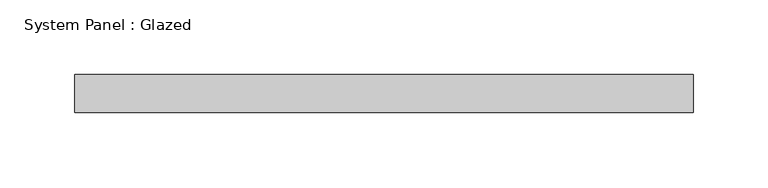
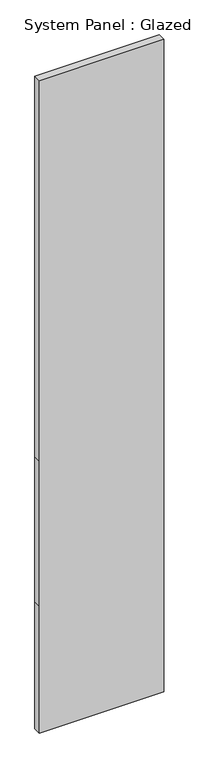
"""IFC4 building model written with IfcOpenShell, lengths in millimetres: plate geometry, System Panel : Glazed."""

from ifc_helpers import new_model, si_unit, frame, origin, place, context, project, spatial, polyline, outline, extrude, source, transform, mapped, element, save


def system_panel_glazed_01ea813e(model_context):
    return source(origin(), model_context, "Body", "SweptSolid", [
        extrude(outline(polyline([(0.0, -206.375), (0.0, 206.375), (444.5, 206.375), (952.5, 206.375), (2286.0, 206.375), (2286.0, -206.375), (952.5, -206.375), (444.5, -206.375), (0.0, -206.375)])), frame((0.0, 19.05, 0.0), z_axis=(0.0, 1.0, 0.0), x_axis=(0.0, 0.0, 1.0)), (0.0, 0.0, 1.0), 25.4),
    ])


if __name__ == "__main__":
    model = new_model("IFC4")
    model_context = context("Model", 3, world=origin())
    ifc_project = project(units=[si_unit("LENGTHUNIT", "METRE", prefix="MILLI")], contexts=[model_context])
    site = spatial("IfcSite", under=ifc_project)
    building = spatial("IfcBuilding", under=site)
    placement = place(None, origin())
    system_panel_glazed_shape = system_panel_glazed_01ea813e(model_context)
    element("IfcPlate", 1, ObjectType="System Panel : Glazed", at=placement, inside=building, context=model_context, shape_type="MappedRepresentation", body=[
        mapped(system_panel_glazed_shape, transform((0.0, 0.0, 0.0), x_axis=(1.0, 0.0, 0.0), y_axis=(0.0, 1.0, 0.0), z_axis=(0.0, 0.0, 1.0))),
    ])
    save(model, "model.ifc")

# Revit data of these elements
# Type "System Panel : Glazed"
#   Construction Type Id = "GSP4R"
#   Analytic Construction = "1/8 in Pilkington single glazing"
#   Visual Light Transmittance = 0.9
#   Solar Heat Gain Coefficient = 0.86
#   Heat Transfer Coefficient (U) = 1.18115 BTU/(h·ft²·°F)
#   Define Thermal Properties by = 1
# Element 1 (IfcPlate, "System Panel : Glazed")
#   Materials on its faces: "Glass"
# Materials
#   "Glass": class "Glass", colour RGB 0 128 192, transparency 0.75, Description = "Soda Lime Glass", Cost = 0
